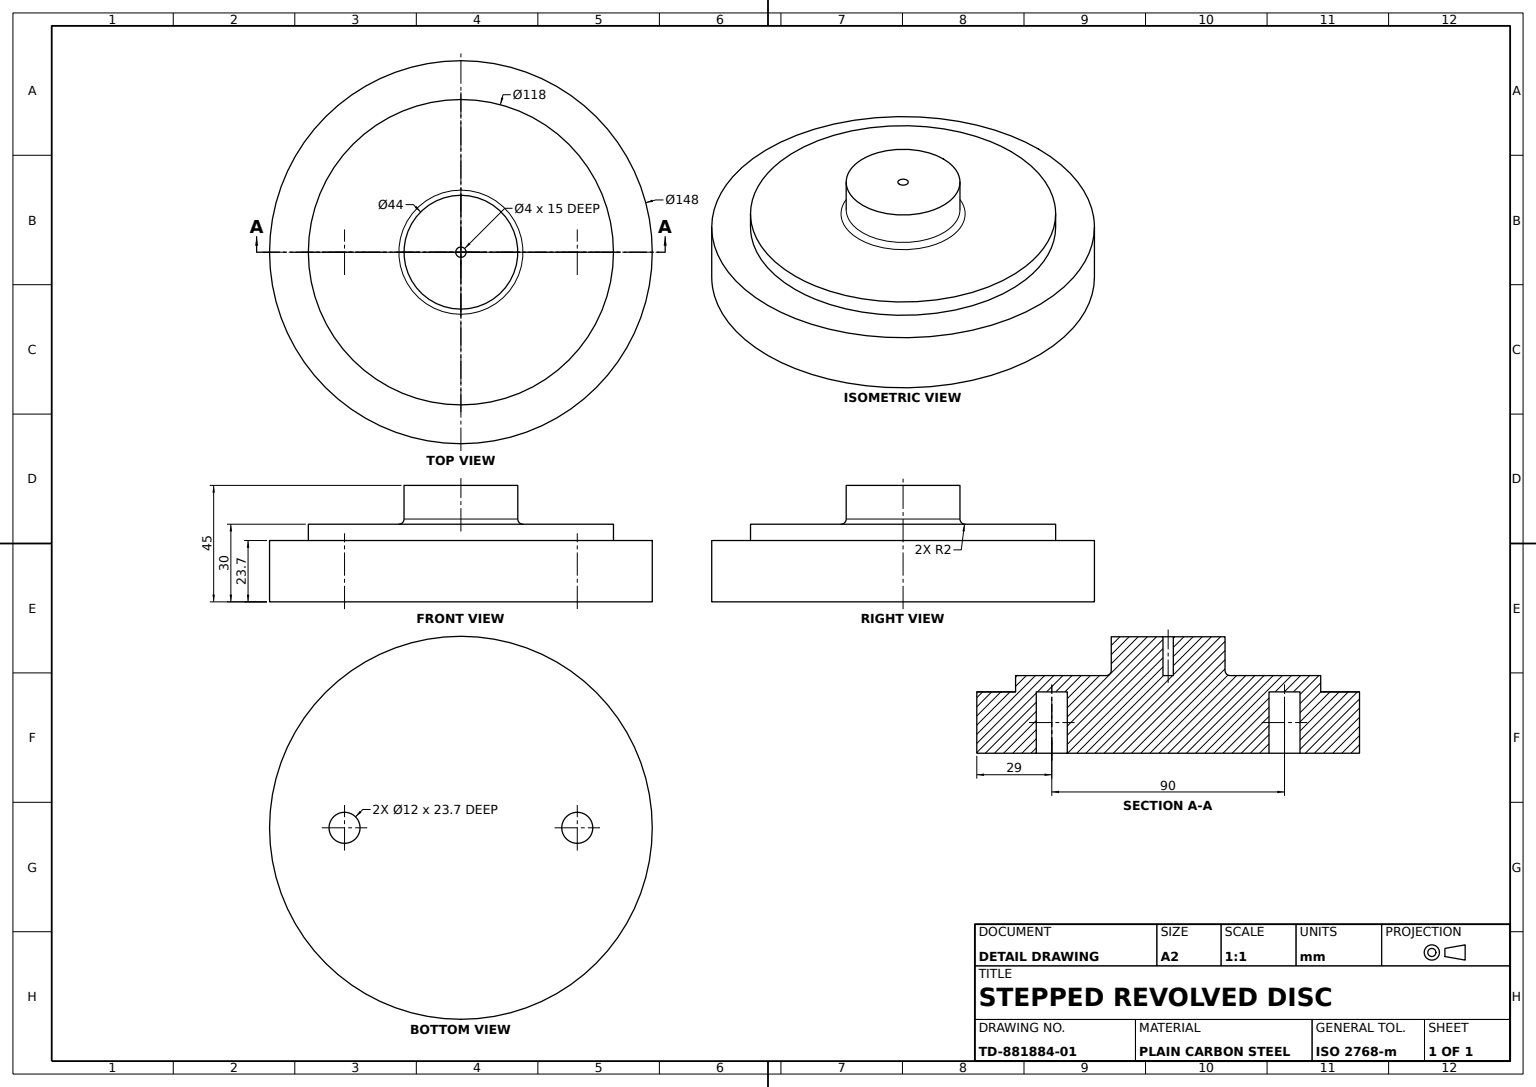
from build123d import *

# Parameters (mm, degrees)
CENTRE_CUT_SKETCH_R = 6
CENTRE_CUT_DEPTH    = 108.301863917


with BuildPart() as part:
    # Disc Profile Sketch → Stepped Disc Revolve (revolve)
    with BuildSketch(Plane.XY, mode=Mode.PRIVATE) as stepped_disc_revolve_sk:
        with BuildLine():
            Line((0, 0), (0, 30))
            Line((0, 30), (2, 30))
            Line((2, 30), (2, 45))
            Line((2, 45), (22, 45))
            Line((22, 45), (22, 32))
            ThreePointArc((22, 32), (22.585786438, 30.585786438), (24, 30))
            Line((24, 30), (59, 30))
            Line((59, 30), (59, 23.7))
            Line((59, 23.7), (74, 23.7))
            Line((74, 23.7), (74, 0))
            Line((74, 0), (0, 0))
        make_face()
    revolve(stepped_disc_revolve_sk.sketch.rotate(Axis((0, 0, 0), (0, 1, 0)), 90), axis=Axis((0, 0, 0), (0, 1, 0)))

    # Centre Cut Sketch → Centre Cut (cut, through all)
    with BuildSketch(Plane(origin=(0, 23.7, 0), x_dir=(1, 0, 0), z_dir=(0, 1, 0))):
        with Locations(Location((-45, 0, 0), (0, 0, 270))):
            Circle(CENTRE_CUT_SKETCH_R)
        with Locations(Location((45, 0, 0), (0, 0, 270))):
            Circle(CENTRE_CUT_SKETCH_R)
    extrude(amount=-CENTRE_CUT_DEPTH, mode=Mode.SUBTRACT)


solid = part.part
